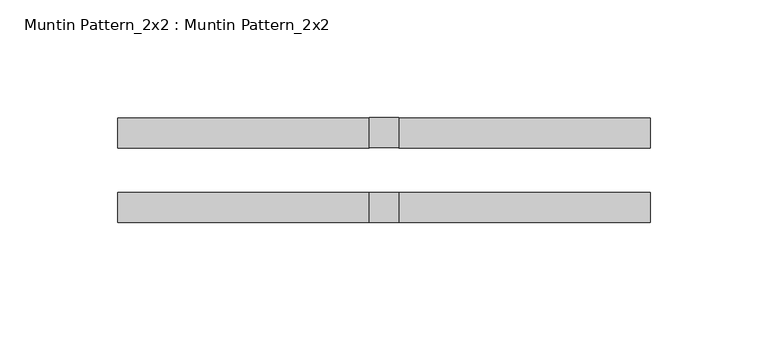
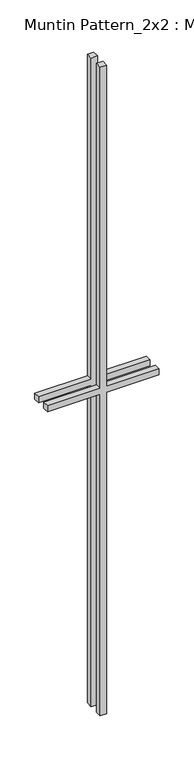
"""IFC4 building model written with IfcOpenShell, lengths in millimetres: proxy geometry, Muntin Pattern_2x2 : Muntin Pattern_2x2."""

from ifc_helpers import new_model, si_unit, frame, origin, place, context, project, spatial, polyline, outline, extrude, source, transform, mapped, element, save


def muntin_pattern_2x2_muntin_pattern_2x2_79566686(model_context):
    return source(origin(), model_context, "Body", "SweptSolid", [
        extrude(outline(polyline([(698.5, -6.35), (698.5, -112.8914087), (685.8, -112.8914087), (685.8, -6.35), (0.0, -6.35), (0.0, 6.35), (685.8, 6.35), (685.8, 112.8914087), (698.5, 112.8914087), (698.5, 6.35), (1384.3, 6.35), (1384.3, -6.35), (698.5, -6.35)])), frame((0.0, 9.525, 0.0), z_axis=(0.0, 1.0, 0.0), x_axis=(0.0, 0.0, 1.0)), (0.0, 0.0, 1.0), 12.7),
        extrude(outline(polyline([(698.5, -6.35), (698.5, -112.8914087), (685.8, -112.8914087), (685.8, -6.35), (0.0, -6.35), (0.0, 6.35), (685.8, 6.35), (685.8, 112.8914087), (698.5, 112.8914087), (698.5, 6.35), (1384.3, 6.35), (1384.3, -6.35), (698.5, -6.35)])), frame((0.0, -22.225, 0.0), z_axis=(0.0, 1.0, 0.0), x_axis=(0.0, 0.0, 1.0)), (0.0, 0.0, 1.0), 12.7),
    ])


if __name__ == "__main__":
    model = new_model("IFC4")
    model_context = context("Model", 3, world=origin())
    ifc_project = project(units=[si_unit("LENGTHUNIT", "METRE", prefix="MILLI")], contexts=[model_context])
    site = spatial("IfcSite", under=ifc_project)
    building = spatial("IfcBuilding", under=site)
    placement = place(None, origin())
    muntin_pattern_2x2_muntin_pattern_2x2_shape = muntin_pattern_2x2_muntin_pattern_2x2_79566686(model_context)
    element("IfcBuildingElementProxy", 1, Name="Muntin Pattern_2x2 : Muntin Pattern_2x2", ObjectType="Muntin Pattern_2x2 : Muntin Pattern_2x2", at=placement, inside=building, context=model_context, shape_type="MappedRepresentation", body=[
        mapped(muntin_pattern_2x2_muntin_pattern_2x2_shape, transform((0.0, 0.0, 0.0), x_axis=(1.0, 0.0, 0.0), y_axis=(0.0, 1.0, 0.0), z_axis=(0.0, 0.0, 1.0))),
    ])
    save(model, "model.ifc")

# Revit data of these elements
# Type "Muntin Pattern_2x2 : Muntin Pattern_2x2"
#   Width [instance default] = 4' - 0"
#   Thickness = 0' - 0 1/2"
#   Height [instance default] = 4' - 0"
#   Distance = 0' - 0 3/4"
#   Interior Material [instance default] = none
#   Exterior Material [instance default] = none
#   Default Elevation = 0
# Element 1 (IfcBuildingElementProxy, "Muntin Pattern_2x2 : Muntin Pattern_2x2")
#   Width = 0' - 8.88909"
#   Height = 4' - 6 1/2"
#   Interior Material = Wood - Stained
#   Exterior Material = Clad - White
#   Materials on its faces: "Clad - White", "Wood - Stained"
# Materials
#   "Clad - White": class "Wood", colour RGB 242 242 238, transparency 0, Cost = 0
#   "Wood - Stained": class "Wood", colour RGB 224 178 126, transparency 0, Cost = 0
